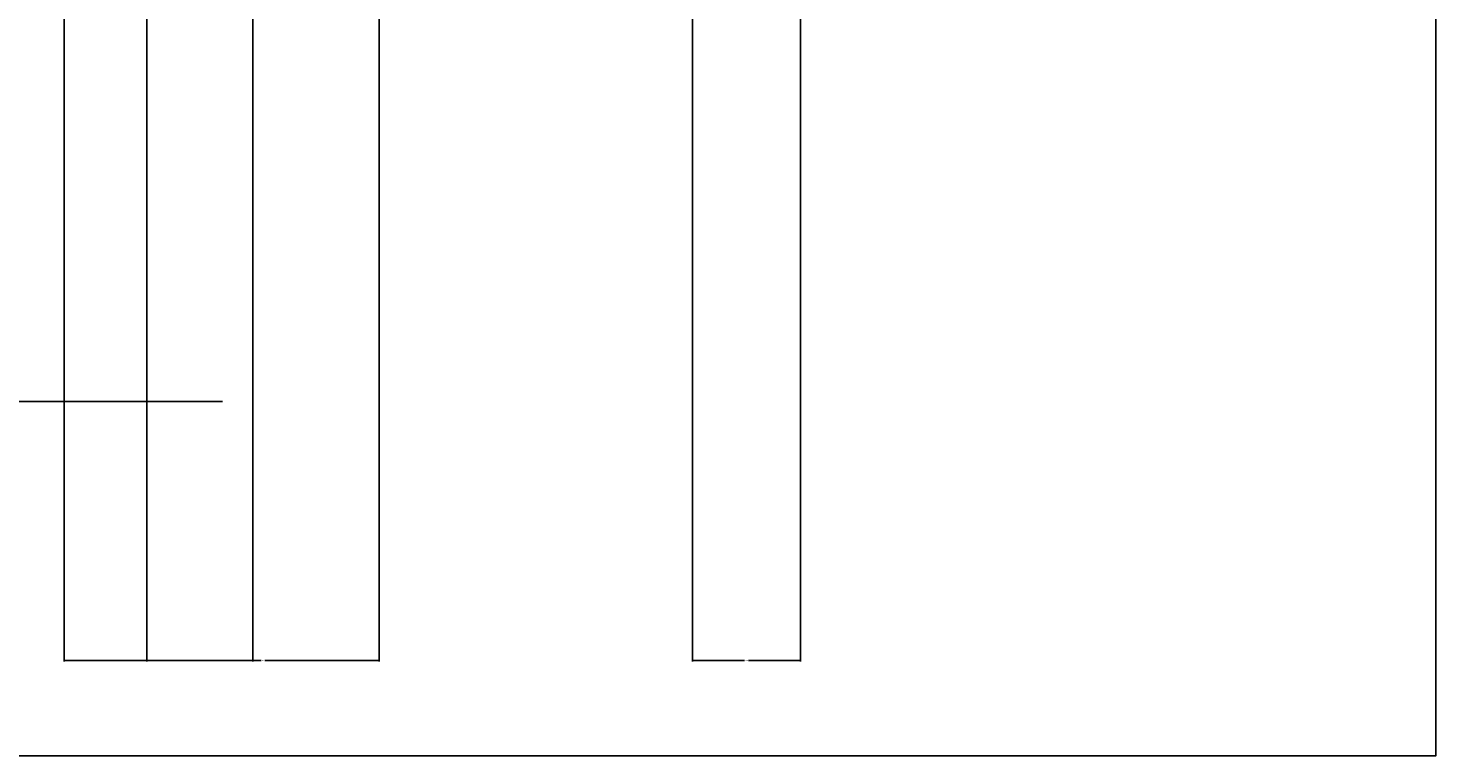
# Model space of a CAD drawing. Units: inches. Extents: x 1601 to 2297, y 1496 to 2631.
# Tile 16 of 57: x 2033 to 2297, y 1496 to 1632. Entities that reach past the tile are written whole.
import ezdxf

# ---------------------------------------------------------------- set-up
doc = ezdxf.new("R2010")
doc.units = ezdxf.units.IN
for name, color, linetype, lineweight in [('A-ANNO-DIMS', 2, 'Continuous', 18), ('A-ANNO-TTLB', 7, 'Continuous', 25), ('A-WALL-PATT', 215, 'Continuous', 13)]:
    doc.layers.add(name, color=color, linetype=linetype, lineweight=lineweight)
doc.styles.get("Standard").update_dxf_attribs({"font": 'arial.ttf'})
doc.dimstyles.get("Standard").update_dxf_attribs({"dimtxt": 0.18, "dimasz": 0.18, "dimexe": 0.18, "dimexo": 0.0625, "dimgap": 0.09, "dimtad": 0, "dimtih": 1, "dimtoh": 1, "dimdec": 4, "dimzin": 0, "dimdsep": 46, "dimtxsty": 'Standard', "dimcen": 0.09, "dimadec": 0, "dimazin": 0, "dimtfac": 1, "dimtdec": 4, "dimtofl": 0, "dimtmove": 0, "dimatfit": 3, "dimfxl": 1, "dimtolj": 1, "dimtzin": 0, "dimarcsym": 0})

# ---------------------------------------------------------------- blocks, each defined once
blk = doc.blocks.new('*D38')
at = {"layer": 'A-ANNO-DIMS', "color": 0, "lineweight": -2, "transparency": 16777216}
for p, q in [((2178.04, 2085.26), (2178.04, 1513.75)), ((2157.8, 2066.51), (2157.8, 1513.75)), ((2157.98, 1513.93), (2167.52, 1513.93)), ((2177.86, 1513.93), (2168.31, 1513.93))]:
    blk.add_line(p, q, dxfattribs=at)
at = {"layer": 'A-ANNO-DIMS', "color": 0, "transparency": 16777216}
for points in [[(2157.98, 1513.96), (2157.98, 1513.9), (2157.8, 1513.93)], [(2177.86, 1513.96), (2177.86, 1513.9), (2178.04, 1513.93)]]:
    blk.add_solid(points, dxfattribs=at)
at = {"layer": 'Defpoints', "color": 0, "transparency": 16777216}
for p in [(2178.04, 2085.33), (2157.8, 2066.58), (2178.04, 1513.93)]:
    blk.add_point(p, dxfattribs=at)
at = {"layer": 'A-ANNO-DIMS', "color": 0, "transparency": 16777216, "insert": (2167.92, 1513.93), "char_height": 0.18, "attachment_point": 5}
blk.add_mtext('\\A1;20.24', dxfattribs=at)
blk = doc.blocks.new('*D39')
at = {"layer": 'A-ANNO-DIMS', "color": 0, "lineweight": -2, "transparency": 16777216}
for p, q in [((2055.55, 1981.76), (2055.55, 1513.75)), ((2099.05, 1981.76), (2099.05, 1513.75)), ((2055.73, 1513.93), (2076.97, 1513.93)), ((2098.87, 1513.93), (2077.63, 1513.93))]:
    blk.add_line(p, q, dxfattribs=at)
at = {"layer": 'A-ANNO-DIMS', "color": 0, "transparency": 16777216}
for points in [[(2055.73, 1513.96), (2055.73, 1513.9), (2055.55, 1513.93)], [(2098.87, 1513.96), (2098.87, 1513.9), (2099.05, 1513.93)]]:
    blk.add_solid(points, dxfattribs=at)
at = {"layer": 'Defpoints', "color": 0, "transparency": 16777216}
for p in [(2055.55, 1981.83), (2099.05, 1981.83), (2099.05, 1513.93)]:
    blk.add_point(p, dxfattribs=at)
at = {"layer": 'A-ANNO-DIMS', "color": 0, "transparency": 16777216, "insert": (2077.3, 1513.93), "char_height": 0.18, "attachment_point": 5}
blk.add_mtext('\\A1;43.5', dxfattribs=at)
blk = doc.blocks.new('*D41')
at = {"layer": 'A-ANNO-DIMS', "color": 0, "lineweight": -2, "transparency": 16777216}
for p, q in [((2075.4, 2070.14), (2075.4, 1513.75)), ((2040.04, 2066.51), (2040.04, 1513.75)), ((2040.22, 1513.93), (2057.32, 1513.93)), ((2075.22, 1513.93), (2058.11, 1513.93))]:
    blk.add_line(p, q, dxfattribs=at)
at = {"layer": 'A-ANNO-DIMS', "color": 0, "transparency": 16777216}
for points in [[(2040.22, 1513.96), (2040.22, 1513.9), (2040.04, 1513.93)], [(2075.22, 1513.96), (2075.22, 1513.9), (2075.4, 1513.93)]]:
    blk.add_solid(points, dxfattribs=at)
at = {"layer": 'Defpoints', "color": 0, "transparency": 16777216}
for p in [(2075.4, 2070.2), (2040.04, 2066.58), (2075.4, 1513.93)]:
    blk.add_point(p, dxfattribs=at)
at = {"layer": 'A-ANNO-DIMS', "color": 0, "transparency": 16777216, "insert": (2057.72, 1513.93), "char_height": 0.18, "attachment_point": 5}
blk.add_mtext('\\A1;35.36', dxfattribs=at)

msp = doc.modelspace()

# ---------------------------------------------------------------- hatches: boundary and pattern name
at = {"layer": 'A-WALL-PATT'}
h = msp.add_hatch(dxfattribs=at)
h.set_pattern_fill('ANSI32', color=256)
h.paths.add_polyline_path([(1842.0336, 2528.0767), (1842.0336, 2532.3254), (1686.0373, 2532.3254), (1686.0373, 2492.9493), (1695.0373, 2492.9493), (1695.0373, 2523.3254), (1827.0373, 2523.3254), (1827.0373, 2416.8254), (1834.6225, 2416.8254), (1834.6225, 2419.0754), (1834.6225, 2421.3254), (1831.5373, 2421.3254), (1831.5373, 2523.3254), (1842.0336, 2523.3254)])
h.paths.add_polyline_path([(1695.0373, 2432.9493), (1686.0373, 2432.9493), (1686.0373, 2325.989), (1695.0373, 2325.989), (1695.0373, 2347.8254), (1827.0373, 2347.8254), (1827.0373, 2287.8254), (1823.2991, 2287.8254), (1823.2991, 2283.3254), (1847.9422, 2283.3254), (1847.9422, 2285.5754), (1847.9422, 2287.8254), (1831.5373, 2287.8254), (1831.5373, 2347.8254), (1846.9946, 2347.8254), (1846.9946, 2350.0754), (1846.9946, 2352.3254), (1695.0373, 2352.3254)])
h.paths.add_polyline_path([(1807.1169, 1573.5395), (2055.0405, 1573.5395), (2055.0405, 1610.6322), (1807.1169, 1610.6322)], flags=9)
h.paths.add_polyline_path([(1841.1631, 1712.7967), (1870.3957, 1712.7967), (1870.3957, 1731.454), (1841.1631, 1731.454)], flags=9)
h.paths.add_polyline_path([(2144.3862, 1772.185), (2191.0233, 1772.185), (2191.0233, 1790.8423), (2144.3862, 1790.8423)], flags=9)
h.paths.add_polyline_path([(2143.0128, 1827.3312), (2177.9958, 1827.3312), (2177.9958, 1845.9886), (2143.0128, 1845.9886)], flags=9)
h.paths.add_polyline_path([(2041.2439, 1833.5691), (2070.8516, 1833.5691), (2070.8516, 1852.2264), (2041.2439, 1852.2264)], flags=9)
h.paths.add_polyline_path([(2097.2791, 1947.0598), (2134.2061, 1947.0598), (2134.2061, 1965.7171), (2097.2791, 1965.7171)], flags=9)
h.paths.add_polyline_path([(2214.995, 1904.3124), (2214.995, 1942.2899), (2196.3376, 1942.2899), (2196.3376, 1904.3124)], flags=9)
h.paths.add_polyline_path([(2186.6284, 2043.8031), (2219.7935, 2043.8031), (2219.7935, 2062.4605), (2186.6284, 2062.4605)], flags=9)
h.paths.add_polyline_path([(2064.0877, 2031.616), (2097.4949, 2031.616), (2097.4949, 2050.2734), (2064.0877, 2050.2734)], flags=9)
h.paths.add_polyline_path([(1973.1349, 1986.0688), (2008.4009, 1986.0688), (2008.4009, 2004.7261), (1973.1349, 2004.7261)], flags=9)
h.paths.add_polyline_path([(1976.3676, 2106.9635), (2005.7469, 2106.9635), (2005.7469, 2125.6209), (1976.3676, 2125.6209)], flags=9)
h.paths.add_polyline_path([(1991.7852, 2180.4863), (2027.0513, 2180.4863), (2027.0513, 2199.1437), (1991.7852, 2199.1437)], flags=9)
h.paths.add_polyline_path([(2106.1801, 2187.9359), (2152.2101, 2187.9359), (2152.2101, 2206.5932), (2106.1801, 2206.5932)], flags=9)
h.paths.add_polyline_path([(2148.6686, 2262.2542), (2182.318, 2262.2542), (2182.318, 2280.9115), (2148.6686, 2280.9115)], flags=9)
h.paths.add_polyline_path([(2041.6327, 2252.8147), (2071.2405, 2252.8147), (2071.2405, 2271.4721), (2041.6327, 2271.4721)], flags=9)
h.paths.add_polyline_path([(2063.9734, 2375.4265), (2100.9004, 2375.4265), (2100.9004, 2394.0839), (2063.9734, 2394.0839)], flags=9)
h.paths.add_polyline_path([(2216.4955, 2330.9748), (2216.4955, 2370.2654), (2197.8381, 2370.2654), (2197.8381, 2330.9748)], flags=9)
h.paths.add_polyline_path([(2179.1416, 2485.8687), (2212.3067, 2485.8687), (2212.3067, 2504.5261), (2179.1416, 2504.5261)], flags=9)
h.paths.add_polyline_path([(2078.7442, 2471.1516), (2112.1514, 2471.1516), (2112.1514, 2489.809), (2078.7442, 2489.809)], flags=9)
h.paths.add_polyline_path([(1915.9631, 2329.4668), (1952.8902, 2329.4668), (1952.8902, 2348.1241), (1915.9631, 2348.1241)], flags=9)
h.paths.add_polyline_path([(1904.3189, 2499.6709), (1940.4512, 2499.6709), (1940.4512, 2518.3282), (1904.3189, 2518.3282)], flags=9)
h.paths.add_polyline_path([(1892.3665, 2100.4595), (1925.6374, 2100.4595), (1925.6374, 2119.1169), (1892.3665, 2119.1169)], flags=9)
h.paths.add_polyline_path([(1909.2984, 1805.9631), (1946.2254, 1805.9631), (1946.2254, 1824.6205), (1909.2984, 1824.6205)], flags=9)
h.paths.add_polyline_path([(1934.6056, 1658.616), (1970.738, 1658.616), (1970.738, 1677.2733), (1934.6056, 1677.2733)], flags=9)
h.paths.add_polyline_path([(1711.2052, 1789.8902), (1750.0456, 1789.8902), (1750.0456, 1808.5476), (1711.2052, 1808.5476)], flags=9)
h.paths.add_polyline_path([(1742.7874, 1854.6743), (1771.9449, 1854.6743), (1771.9449, 1873.3317), (1742.7874, 1873.3317)], flags=9)
h.paths.add_polyline_path([(1807.3592, 1997.7912), (1850.1116, 1997.7912), (1850.1116, 2016.4486), (1807.3592, 2016.4486)], flags=9)
h.paths.add_polyline_path([(1717.4579, 2237.7844), (1760.2103, 2237.7844), (1760.2103, 2256.4417), (1717.4579, 2256.4417)], flags=9)
h.paths.add_polyline_path([(1780.9285, 2324.0623), (1810.086, 2324.0623), (1810.086, 2342.7197), (1780.9285, 2342.7197)], flags=25)
h.paths.add_polyline_path([(1837.696, 2449.2024), (1866.9286, 2449.2024), (1866.9286, 2467.8598), (1837.696, 2467.8598)], flags=9)
h.paths.add_polyline_path([(1712.7752, 2484.9404), (1751.6156, 2484.9404), (1751.6156, 2503.5977), (1712.7752, 2503.5977)], flags=25)
h = msp.add_hatch(dxfattribs=at)
h.set_pattern_fill('ANSI32', color=256)
h.paths.add_polyline_path([(1973.9371, 2211.3254), (1893.0373, 2211.3254), (1893.0373, 2287.8254), (1884.6167, 2287.8254), (1884.6167, 2285.5754), (1884.6167, 2283.3254), (1888.5373, 2283.3254), (1888.5373, 2145.3254), (1695.0373, 2145.3254), (1695.0373, 2173.8724), (1690.5373, 2173.8724), (1686.0373, 2173.8724), (1686.0373, 2136.3254), (1722.5687, 2136.3254), (1722.5687, 2117.4352), (1731.5687, 2117.4352), (1731.5687, 2136.3254), (1893.0373, 2136.3254), (1893.0373, 2202.3254), (1959.0373, 2202.3254), (1959.0373, 2182.1303), (1968.0373, 2182.1303), (1968.0373, 2202.3254), (1973.9371, 2202.3254)])
h.paths.add_polyline_path([(2094.0373, 2274.6364), (2096.4294, 2274.6364), (2096.4294, 2276.8864), (2096.4294, 2279.1364), (2094.0373, 2279.1364), (2094.0373, 2290.8254), (2094.0373, 2295.3254), (2089.5373, 2295.3254), (2089.5373, 2230.8254), (2035.5373, 2230.8254), (2035.5373, 2299.8254), (2031.0373, 2299.8254), (2031.0373, 2211.3254), (2023.0065, 2211.3254), (2023.0065, 2202.3254), (2031.0373, 2202.3254), (2031.0373, 2140.8254), (1968.0373, 2140.8254), (1968.0373, 2145.9106), (1963.5373, 2145.9106), (1959.0373, 2145.9106), (1959.0373, 2116.839), (1963.5373, 2116.839), (1968.0373, 2116.839), (1968.0373, 2131.8254), (2031.0373, 2131.8254), (2031.0373, 2094.3254), (2031.0373, 2085.3254), (2031.0373, 2056.8254), (1968.0373, 2056.8254), (1968.0373, 2070.4947), (1963.5373, 2070.4947), (1959.0373, 2070.4947), (1959.0373, 2040.3029), (1968.0373, 2040.3029), (1968.0373, 2047.8254), (2031.0373, 2047.8254), (2031.0373, 1983.3254), (2031.0373, 1978.8254), (2021.1979, 1978.8254), (2021.1979, 1974.3254), (2031.0373, 1974.3254), (2031.0373, 1954.3528), (2035.5373, 1954.3528), (2035.5373, 1974.3254), (2035.5373, 1981.8254), (2055.5513, 1981.8254), (2055.5513, 1986.3254), (2035.5373, 1986.3254), (2035.5373, 2047.8254), (2040.0373, 2047.8254), (2040.0373, 2085.3254), (2040.0373, 2094.3254), (2040.0373, 2140.8254), (2035.5373, 2140.8254), (2035.5373, 2226.3254), (2089.5373, 2226.3254), (2094.0373, 2226.3254)])
h.paths.add_polyline_path([(2226.0373, 2230.8254), (2134.5373, 2230.8254), (2134.5373, 2233.5437), (2130.0373, 2233.5437), (2130.0373, 2226.3254), (2134.5373, 2226.3254), (2226.0373, 2226.3254)])
h.paths.add_polyline_path([(1807.1169, 1573.5395), (2055.0405, 1573.5395), (2055.0405, 1610.6322), (1807.1169, 1610.6322)], flags=9)
h.paths.add_polyline_path([(1841.1631, 1712.7967), (1870.3957, 1712.7967), (1870.3957, 1731.454), (1841.1631, 1731.454)], flags=9)
h.paths.add_polyline_path([(2144.3862, 1772.185), (2191.0233, 1772.185), (2191.0233, 1790.8423), (2144.3862, 1790.8423)], flags=9)
h.paths.add_polyline_path([(2143.0128, 1827.3312), (2177.9958, 1827.3312), (2177.9958, 1845.9886), (2143.0128, 1845.9886)], flags=9)
h.paths.add_polyline_path([(2041.2439, 1833.5691), (2070.8516, 1833.5691), (2070.8516, 1852.2264), (2041.2439, 1852.2264)], flags=9)
h.paths.add_polyline_path([(2097.2791, 1947.0598), (2134.2061, 1947.0598), (2134.2061, 1965.7171), (2097.2791, 1965.7171)], flags=9)
h.paths.add_polyline_path([(2214.995, 1904.3124), (2214.995, 1942.2899), (2196.3376, 1942.2899), (2196.3376, 1904.3124)], flags=9)
h.paths.add_polyline_path([(2186.6284, 2043.8031), (2219.7935, 2043.8031), (2219.7935, 2062.4605), (2186.6284, 2062.4605)], flags=9)
h.paths.add_polyline_path([(2064.0877, 2031.616), (2097.4949, 2031.616), (2097.4949, 2050.2734), (2064.0877, 2050.2734)], flags=9)
h.paths.add_polyline_path([(1973.1349, 1986.0688), (2008.4009, 1986.0688), (2008.4009, 2004.7261), (1973.1349, 2004.7261)], flags=25)
h.paths.add_polyline_path([(1976.3676, 2106.9635), (2005.7469, 2106.9635), (2005.7469, 2125.6209), (1976.3676, 2125.6209)], flags=25)
h.paths.add_polyline_path([(1991.7852, 2180.4863), (2027.0513, 2180.4863), (2027.0513, 2199.1437), (1991.7852, 2199.1437)], flags=25)
h.paths.add_polyline_path([(2106.1801, 2187.9359), (2152.2101, 2187.9359), (2152.2101, 2206.5932), (2106.1801, 2206.5932)], flags=9)
h.paths.add_polyline_path([(2148.6686, 2262.2542), (2182.318, 2262.2542), (2182.318, 2280.9115), (2148.6686, 2280.9115)], flags=9)
h.paths.add_polyline_path([(2041.6327, 2252.8147), (2071.2405, 2252.8147), (2071.2405, 2271.4721), (2041.6327, 2271.4721)], flags=25)
h.paths.add_polyline_path([(2063.9734, 2375.4265), (2100.9004, 2375.4265), (2100.9004, 2394.0839), (2063.9734, 2394.0839)], flags=9)
h.paths.add_polyline_path([(2216.4955, 2330.9748), (2216.4955, 2370.2654), (2197.8381, 2370.2654), (2197.8381, 2330.9748)], flags=9)
h.paths.add_polyline_path([(2179.1416, 2485.8687), (2212.3067, 2485.8687), (2212.3067, 2504.5261), (2179.1416, 2504.5261)], flags=9)
h.paths.add_polyline_path([(2078.7442, 2471.1516), (2112.1514, 2471.1516), (2112.1514, 2489.809), (2078.7442, 2489.809)], flags=9)
h.paths.add_polyline_path([(1915.9631, 2329.4668), (1952.8902, 2329.4668), (1952.8902, 2348.1241), (1915.9631, 2348.1241)], flags=9)
h.paths.add_polyline_path([(1904.3189, 2499.6709), (1940.4512, 2499.6709), (1940.4512, 2518.3282), (1904.3189, 2518.3282)], flags=9)
h.paths.add_polyline_path([(1892.3665, 2100.4595), (1925.6374, 2100.4595), (1925.6374, 2119.1169), (1892.3665, 2119.1169)], flags=9)
h.paths.add_polyline_path([(1909.2984, 1805.9631), (1946.2254, 1805.9631), (1946.2254, 1824.6205), (1909.2984, 1824.6205)], flags=9)
h.paths.add_polyline_path([(1934.6056, 1658.616), (1970.738, 1658.616), (1970.738, 1677.2733), (1934.6056, 1677.2733)], flags=9)
h.paths.add_polyline_path([(1711.2052, 1789.8902), (1750.0456, 1789.8902), (1750.0456, 1808.5476), (1711.2052, 1808.5476)], flags=9)
h.paths.add_polyline_path([(1742.7874, 1854.6743), (1771.9449, 1854.6743), (1771.9449, 1873.3317), (1742.7874, 1873.3317)], flags=9)
h.paths.add_polyline_path([(1807.3592, 1997.7912), (1850.1116, 1997.7912), (1850.1116, 2016.4486), (1807.3592, 2016.4486)], flags=9)
h.paths.add_polyline_path([(1717.4579, 2237.7844), (1760.2103, 2237.7844), (1760.2103, 2256.4417), (1717.4579, 2256.4417)], flags=25)
h.paths.add_polyline_path([(1780.9285, 2324.0623), (1810.086, 2324.0623), (1810.086, 2342.7197), (1780.9285, 2342.7197)], flags=9)
h.paths.add_polyline_path([(1837.696, 2449.2024), (1866.9286, 2449.2024), (1866.9286, 2467.8598), (1837.696, 2467.8598)], flags=9)
h.paths.add_polyline_path([(1712.7752, 2484.9404), (1751.6156, 2484.9404), (1751.6156, 2503.5977), (1712.7752, 2503.5977)], flags=9)
h = msp.add_hatch(dxfattribs=at)
h.set_pattern_fill('ANSI32', color=256)
h.paths.add_polyline_path([(2230.5373, 1861.8254), (2182.5373, 1861.8254), (2182.5373, 1885.3637), (2178.0373, 1885.3637), (2178.0373, 1861.8254), (2166.0373, 1861.8254), (2134.5373, 1861.8254), (2130.0373, 1861.8254), (2130.0373, 1841.4682), (2126.8833, 1841.4682), (2126.8833, 1836.9682), (2130.0373, 1836.9682), (2130.0373, 1822.7302), (2134.5373, 1822.7302), (2134.5373, 1857.3254), (2166.0373, 1857.3254), (2226.0373, 1857.3254), (2226.0373, 1846.1155), (2230.5373, 1846.1155)])
h.paths.add_polyline_path([(2226.0373, 1797.3254), (2134.5373, 1797.3254), (2134.5373, 1800.6636), (2132.2873, 1800.6636), (2130.0373, 1800.6636), (2130.0373, 1797.3254), (2130.0373, 1792.8254), (2167.7264, 1792.8254), (2226.0373, 1792.8254)])
h.paths.add_polyline_path([(2230.5373, 1822.1155), (2226.0373, 1822.1155), (2226.0373, 1760.8563), (2230.5373, 1760.8563)])
h.paths.add_polyline_path([(2230.5373, 1700.8563), (2226.0373, 1700.8563), (2226.0373, 1644.3254), (2140.2517, 1644.3254), (2140.2517, 1635.3254), (2230.5373, 1635.3254)])
h.paths.add_polyline_path([(2080.2517, 1639.8254), (2080.2517, 1644.3254), (2035.5373, 1644.3254), (2035.5373, 1792.8254), (2094.0373, 1792.8254), (2094.0373, 1797.3254), (2094.0373, 1836.9682), (2097.1057, 1836.9682), (2097.1057, 1839.2182), (2097.1057, 1841.4682), (2094.0373, 1841.4682), (2094.0373, 1862.2276), (2089.5373, 1862.2276), (2089.5373, 1797.3254), (2035.5373, 1797.3254), (2035.5373, 1857.3254), (2035.5373, 1885.0916), (2031.0373, 1885.0916), (2031.0373, 1710.3254), (2012.329, 1710.3254), (2012.329, 1701.3254), (2031.0373, 1701.3254), (2031.0373, 1644.3254), (2031.0373, 1635.3254), (2080.2517, 1635.3254)])
h.paths.add_polyline_path([(1836.0373, 1653.2033), (1842.6171, 1653.2033), (1842.6171, 1657.7033), (1842.6171, 1662.2033), (1831.5373, 1662.2033), (1831.5373, 1764.2033), (1835.3881, 1764.2033), (1835.3881, 1766.4533), (1835.3881, 1768.7033), (1831.5373, 1768.7033), (1827.0373, 1768.7033), (1827.0373, 1662.2033), (1827.0373, 1635.3254), (1836.0373, 1635.3254)])
h.paths.add_polyline_path([(1893.0373, 1701.3254), (1907.193, 1701.3254), (1907.193, 1705.8254), (1907.193, 1710.3254), (1893.0373, 1710.3254), (1893.0373, 1819.8254), (1882.6444, 1819.8254), (1882.6444, 1817.5754), (1882.6444, 1815.3254), (1888.5373, 1815.3254), (1888.5373, 1662.2033), (1884.0373, 1662.2033), (1866.6171, 1662.2033), (1866.6171, 1653.2033), (1882.391, 1653.2033), (1884.0373, 1653.2033), (1884.0373, 1635.3254), (1893.0373, 1635.3254)])
h.paths.add_polyline_path([(1739.3335, 1639.8254), (1739.3335, 1644.3254), (1695.0373, 1644.3254), (1695.0373, 1702.0135), (1690.5373, 1702.0135), (1686.0373, 1702.0135), (1686.0373, 1635.3254), (1739.3335, 1635.3254)])
h.paths.add_polyline_path([(1827.0373, 1644.3254), (1799.3335, 1644.3254), (1799.3335, 1635.3254), (1827.0373, 1635.3254)])
h.paths.add_polyline_path([(1695.0373, 1815.3254), (1849.2759, 1815.3254), (1849.2759, 1819.8254), (1807.5373, 1819.8254), (1807.5373, 1879.8254), (1851.1533, 1879.8254), (1851.1533, 1882.0754), (1851.1533, 1884.3254), (1799.3405, 1884.3254), (1799.3405, 1882.0754), (1799.3405, 1879.8254), (1803.0373, 1879.8254), (1803.0373, 1819.8254), (1695.0373, 1819.8254), (1695.0373, 1835.0458), (1690.5373, 1835.0458), (1686.0373, 1835.0458), (1686.0373, 1766.1753), (1695.0373, 1766.1753)])
h.paths.add_polyline_path([(1775.8157, 1884.3254), (1695.0373, 1884.3254), (1695.0373, 1912.9526), (1690.5373, 1912.9526), (1686.0373, 1912.9526), (1686.0373, 1859.0458), (1695.0373, 1859.0458), (1695.0373, 1879.8254), (1775.8157, 1879.8254)])
h.paths.add_polyline_path([(1893.0373, 2031.3254), (1731.5687, 2031.3254), (1731.5687, 2057.4352), (1722.5687, 2057.4352), (1722.5687, 2031.3254), (1686.0373, 2031.3254), (1686.0373, 1972.9526), (1695.0373, 1972.9526), (1695.0373, 2022.3254), (1888.5373, 2022.3254), (1888.5373, 1884.3254), (1883.4996, 1884.3254), (1883.4996, 1879.8254), (1893.0373, 1879.8254), (1893.0373, 1974.3254), (1976.6199, 1974.3254), (1976.6199, 1978.8254), (1968.0373, 1978.8254), (1968.0373, 1983.3254), (1968.0373, 2008.4756), (1963.5373, 2008.4756), (1959.0373, 2008.4756), (1959.0373, 1983.3254), (1893.0373, 1983.3254)])
h.paths.add_polyline_path([(2230.5373, 2140.4745), (2226.0373, 2140.4745), (2226.0373, 2094.3254), (2040.0373, 2094.3254), (2040.0373, 2085.3254), (2178.0373, 2085.3254), (2178.0373, 2065.6965), (2182.5373, 2065.6965), (2182.5373, 2085.3254), (2226.0373, 2085.3254), (2226.0373, 1986.3254), (2211.2679, 1986.3254), (2211.2679, 1981.8254), (2230.5373, 1981.8254)])
h.paths.add_polyline_path([(2187.6292, 1986.3254), (2182.5373, 1986.3254), (2182.5373, 2029.6965), (2178.0373, 2029.6965), (2178.0373, 1986.3254), (2099.05, 1986.3254), (2099.05, 1981.8254), (2178.0373, 1981.8254), (2178.0373, 1969.3637), (2182.5373, 1969.3637), (2182.5373, 1981.8254), (2187.6292, 1981.8254), (2187.6292, 1984.0754)])
h.paths.add_polyline_path([(1807.1169, 1573.5395), (2055.0405, 1573.5395), (2055.0405, 1610.6322), (1807.1169, 1610.6322)], flags=9)
h.paths.add_polyline_path([(1841.1631, 1712.7967), (1870.3957, 1712.7967), (1870.3957, 1731.454), (1841.1631, 1731.454)], flags=9)
h.paths.add_polyline_path([(2144.3862, 1772.185), (2191.0233, 1772.185), (2191.0233, 1790.8423), (2144.3862, 1790.8423)], flags=9)
h.paths.add_polyline_path([(2143.0128, 1827.3312), (2177.9958, 1827.3312), (2177.9958, 1845.9886), (2143.0128, 1845.9886)], flags=25)
h.paths.add_polyline_path([(2041.2439, 1833.5691), (2070.8516, 1833.5691), (2070.8516, 1852.2264), (2041.2439, 1852.2264)], flags=25)
h.paths.add_polyline_path([(2097.2791, 1947.0598), (2134.2061, 1947.0598), (2134.2061, 1965.7171), (2097.2791, 1965.7171)], flags=9)
h.paths.add_polyline_path([(2214.995, 1904.3124), (2214.995, 1942.2899), (2196.3376, 1942.2899), (2196.3376, 1904.3124)], flags=9)
h.paths.add_polyline_path([(2186.6284, 2043.8031), (2219.7935, 2043.8031), (2219.7935, 2062.4605), (2186.6284, 2062.4605)], flags=25)
h.paths.add_polyline_path([(2064.0877, 2031.616), (2097.4949, 2031.616), (2097.4949, 2050.2734), (2064.0877, 2050.2734)], flags=25)
h.paths.add_polyline_path([(1973.1349, 1986.0688), (2008.4009, 1986.0688), (2008.4009, 2004.7261), (1973.1349, 2004.7261)], flags=9)
h.paths.add_polyline_path([(1976.3676, 2106.9635), (2005.7469, 2106.9635), (2005.7469, 2125.6209), (1976.3676, 2125.6209)], flags=9)
h.paths.add_polyline_path([(1991.7852, 2180.4863), (2027.0513, 2180.4863), (2027.0513, 2199.1437), (1991.7852, 2199.1437)], flags=9)
h.paths.add_polyline_path([(2106.1801, 2187.9359), (2152.2101, 2187.9359), (2152.2101, 2206.5932), (2106.1801, 2206.5932)], flags=9)
h.paths.add_polyline_path([(2148.6686, 2262.2542), (2182.318, 2262.2542), (2182.318, 2280.9115), (2148.6686, 2280.9115)], flags=9)
h.paths.add_polyline_path([(2041.6327, 2252.8147), (2071.2405, 2252.8147), (2071.2405, 2271.4721), (2041.6327, 2271.4721)], flags=9)
h.paths.add_polyline_path([(2063.9734, 2375.4265), (2100.9004, 2375.4265), (2100.9004, 2394.0839), (2063.9734, 2394.0839)], flags=9)
h.paths.add_polyline_path([(2216.4955, 2330.9748), (2216.4955, 2370.2654), (2197.8381, 2370.2654), (2197.8381, 2330.9748)], flags=9)
h.paths.add_polyline_path([(2179.1416, 2485.8687), (2212.3067, 2485.8687), (2212.3067, 2504.5261), (2179.1416, 2504.5261)], flags=9)
h.paths.add_polyline_path([(2078.7442, 2471.1516), (2112.1514, 2471.1516), (2112.1514, 2489.809), (2078.7442, 2489.809)], flags=9)
h.paths.add_polyline_path([(1915.9631, 2329.4668), (1952.8902, 2329.4668), (1952.8902, 2348.1241), (1915.9631, 2348.1241)], flags=9)
h.paths.add_polyline_path([(1904.3189, 2499.6709), (1940.4512, 2499.6709), (1940.4512, 2518.3282), (1904.3189, 2518.3282)], flags=9)
h.paths.add_polyline_path([(1892.3665, 2100.4595), (1925.6374, 2100.4595), (1925.6374, 2119.1169), (1892.3665, 2119.1169)], flags=9)
h.paths.add_polyline_path([(1909.2984, 1805.9631), (1946.2254, 1805.9631), (1946.2254, 1824.6205), (1909.2984, 1824.6205)], flags=9)
h.paths.add_polyline_path([(1934.6056, 1658.616), (1970.738, 1658.616), (1970.738, 1677.2733), (1934.6056, 1677.2733)], flags=9)
h.paths.add_polyline_path([(1711.2052, 1789.8902), (1750.0456, 1789.8902), (1750.0456, 1808.5476), (1711.2052, 1808.5476)], flags=25)
h.paths.add_polyline_path([(1742.7874, 1854.6743), (1771.9449, 1854.6743), (1771.9449, 1873.3317), (1742.7874, 1873.3317)], flags=25)
h.paths.add_polyline_path([(1807.3592, 1997.7912), (1850.1116, 1997.7912), (1850.1116, 2016.4486), (1807.3592, 2016.4486)], flags=25)
h.paths.add_polyline_path([(1717.4579, 2237.7844), (1760.2103, 2237.7844), (1760.2103, 2256.4417), (1717.4579, 2256.4417)], flags=9)
h.paths.add_polyline_path([(1780.9285, 2324.0623), (1810.086, 2324.0623), (1810.086, 2342.7197), (1780.9285, 2342.7197)], flags=9)
h.paths.add_polyline_path([(1837.696, 2449.2024), (1866.9286, 2449.2024), (1866.9286, 2467.8598), (1837.696, 2467.8598)], flags=9)
h.paths.add_polyline_path([(1712.7752, 2484.9404), (1751.6156, 2484.9404), (1751.6156, 2503.5977), (1712.7752, 2503.5977)], flags=9)

# ---------------------------------------------------------------- linework, layer by layer
at = {"layer": 'A-ANNO-TTLB'}
msp.add_line((1781.0743, 1562.4779), (2069.7201, 1562.4779), dxfattribs=at)
msp.add_lwpolyline([(1600.5933, 2631.1477), (2297.129, 2631.1477), (2297.129, 1496.1026), (1600.5933, 1496.1026)], close=True, dxfattribs=at)

# ---------------------------------------------------------------- dimensions: what is measured, and where the dimension line sits
at = {"layer": 'A-ANNO-DIMS'}
for base, p1, p2, override, picture, middle in [((2178.0373, 1513.9279), (2157.799, 2066.5754), (2178.0373, 2085.3254), {"dimdec": 2, "dimlfac": 1, "dimrnd": 0, "dimzin": 0, "dimdsep": 46, "dimlunit": 2}, '*D38', (2167.9181, 1513.9279)), ((2075.3977, 1513.9279), (2040.0373, 2066.5754), (2075.3977, 2070.1988), {"dimdec": 2, "dimlfac": 1, "dimrnd": 0, "dimzin": 0, "dimdsep": 46, "dimlunit": 2}, '*D41', (2057.7175, 1513.9279)), ((2099.05, 1513.9279), (2055.5513, 1981.8254), (2099.05, 1981.8254), {"dimdec": 1, "dimlfac": 1, "dimrnd": 0, "dimzin": 0, "dimdsep": 46, "dimlunit": 2}, '*D39', (2077.3006, 1513.9279))]:
    dim = msp.add_linear_dim(base=base, p1=p1, p2=p2, dimstyle='Standard', override=override, dxfattribs=at)
    dim.commit()
    dim.dimension.update_dxf_attribs({"geometry": picture, "text_midpoint": middle})

doc.saveas('drawing.dxf')
